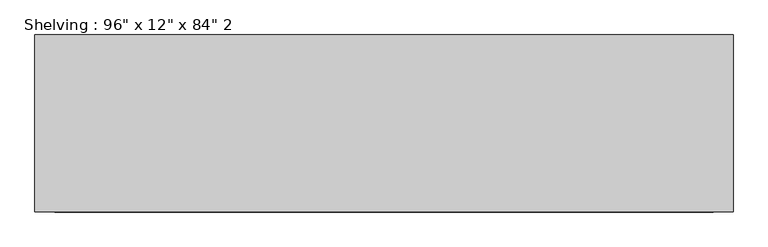
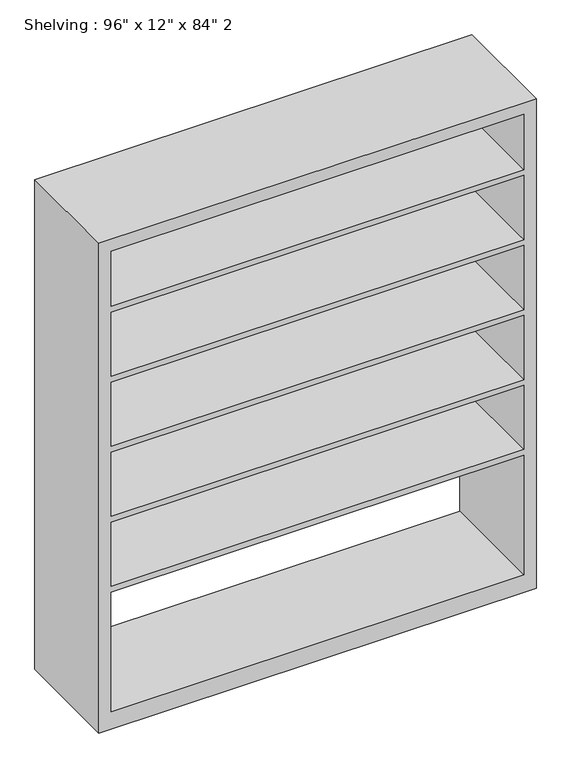
"""IFC4 building model written with IfcOpenShell, lengths in millimetres: furniture geometry."""

from ifc_helpers import new_model, si_unit, frame, origin, place, context, project, spatial, polyline, outline, extrude, source, transform, mapped, element, save


def furniture_df918c0e(model_context):
    return source(origin(), model_context, "Body", "SweptSolid", [
        extrude(outline(polyline([(0.0, 901.7), (2133.6, 901.7), (2133.6, -901.7), (0.0, -901.7), (0.0, 901.7)]), holes=[polyline([(2082.8, 850.9), (1841.5, 850.9), (1841.5, -850.9), (2082.8, -850.9), (2082.8, 850.9)]), polyline([(76.2, 850.9), (76.2, -850.9), (596.9, -850.9), (596.9, 850.9), (76.2, 850.9)]), polyline([(1231.9, -850.9), (1511.3, -850.9), (1511.3, 850.9), (1231.9, 850.9), (1231.9, -850.9)]), polyline([(1816.1, 850.9), (1536.7, 850.9), (1536.7, -850.9), (1816.1, -850.9), (1816.1, 850.9)]), polyline([(1206.5, 850.9), (927.1, 850.9), (927.1, -850.9), (1206.5, -850.9), (1206.5, 850.9)]), polyline([(901.7, 850.9), (622.3, 850.9), (622.3, -850.9), (901.7, -850.9), (901.7, 850.9)])]), frame((0.0, -533.4, 0.0), z_axis=(0.0, 1.0, 0.0), x_axis=(0.0, 0.0, 1.0)), (0.0, 0.0, 1.0), 457.2),
    ])


if __name__ == "__main__":
    model = new_model("IFC4")
    model_context = context("Model", 3, world=origin())
    ifc_project = project(units=[si_unit("LENGTHUNIT", "METRE", prefix="MILLI")], contexts=[model_context])
    site = spatial("IfcSite", under=ifc_project)
    building = spatial("IfcBuilding", under=site)
    placement = place(None, origin())
    furniture_shape = furniture_df918c0e(model_context)
    element("IfcFurniture", 1, ObjectType="Shelving : 96\" x 12\" x 84\" 2", at=placement, inside=building, context=model_context, shape_type="MappedRepresentation", body=[
        mapped(furniture_shape, transform((0.0, 0.0, 0.0), x_axis=(1.0, 0.0, 0.0), y_axis=(0.0, 1.0, 0.0), z_axis=(0.0, 0.0, 1.0))),
    ])
    save(model, "model.ifc")

# Revit data of these elements
# Type "Shelving : 96\" x 12\" x 84\" 2"
#   Assembly Code = "E2020200"
#   Depth = 1' - 6"
#   Height = 7' - 0"
#   Width = 5' - 11"
#   Shelving Unit Material = Laminate, Ivory, Matte
#   Default Elevation = 0
# Element 1 (IfcFurniture, "Shelving : 96\" x 12\" x 84\" 2")
#   Materials on its faces: "Laminate, Ivory, Matte"
# Materials
#   "Laminate, Ivory, Matte": class "Plastic", colour RGB 247 247 239, transparency 0, Description = "Plastic Laminate - Ivory, Matte", Cost = 0
